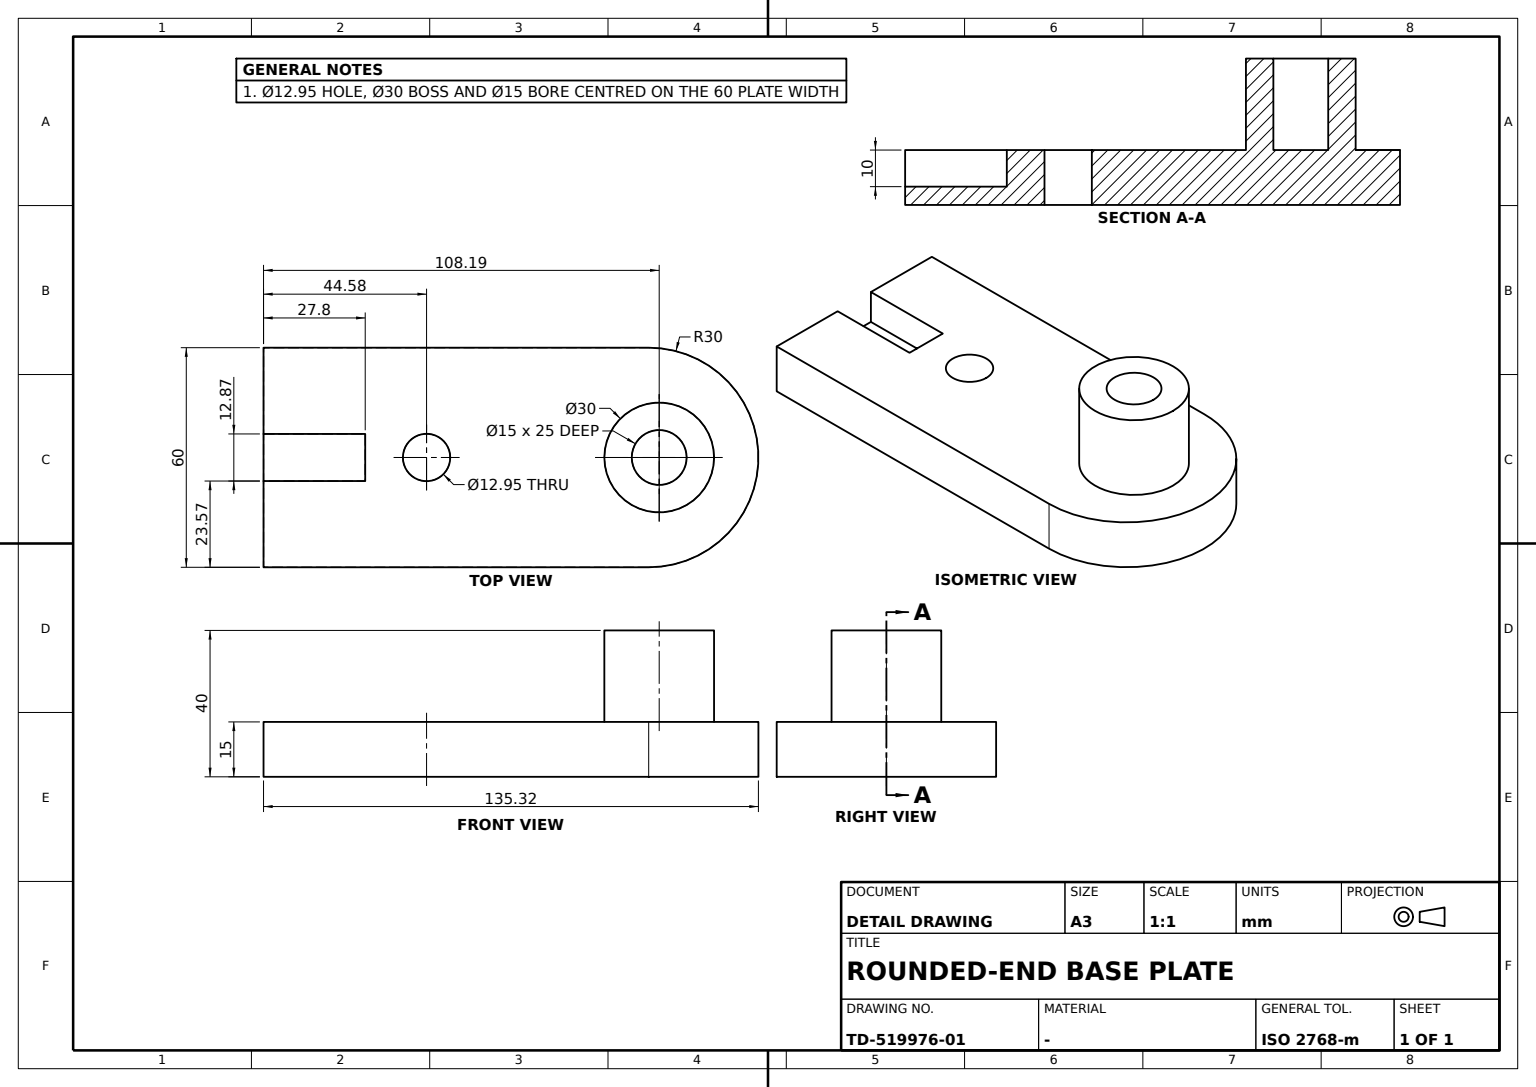
CATIA V5 part; units mm, degrees
sketch "Sketch1" plane through (0, 0, 0) normal (0, 0, 1) x (1, 0, 0)
  line L0 (40.1579, -30) -> (-65.1579, -30)
  line L1 (-65.1579, -30) -> (-65.1579, 30)
  line L2 (-65.1579, 30) -> (40.1579, 30)
  arc A0 (40.1579, 30) -> (40.1579, -30) centre (40.1579, 0) cw
  point P0 (40.1579, 30)
  point P1 (40.1579, -30)
  point P2 (40.1579, -30)
  point P3 (40.1579, 30)
  dimension "length L1" = 60
  constraint horizontal L0 x-axis
  constraint horizontal L2 x-axis
  constraint vertical L1 y-axis
  constraint equidistance L0 L2 origin
  constraint coincidence P0 L2
  constraint coincidence P1 L0
  constraint coincidence P0 P3
  constraint coincidence P1 P2
  constraint tangency A0 L0
extrude "Pad1" add sketch "Sketch1" along normal blind 15
sketch "Sketch2" plane through (0, 0, 15) normal (0, 0, 1) x (1, 0, 0)
  line L0 (43.0311, 28.8591) -> (43.0311, -47.18) construction
  circle A0 centre (43.0311, 0) radius 15
  point P0 (43.0311, 0)
  circle A1 centre (43.0311, 0) radius 7.5
  point P1 (50.5311, 0)
  dimension "radius A0" = 15
  dimension "radius A1" = 7.5
  constraint vertical L0 y-axis
  constraint coincidence P0 L0
  constraint coincidence P0 x-axis
  constraint coincidence A1 P1
  constraint coincidence P1 x-axis
extrude "Pad2" add sketch "Sketch2" along normal blind 25
sketch "Sketch3" plane through (0, 0, 15) normal (0, 0, 1) x (1, 0, 0)
  point P0 (-64.9666, 0)
  line L0 (-37.3555, 6.4328) -> (-37.3555, -6.4328)
  line L1 (-37.3555, -6.4328) -> (-92.5776, -6.4328)
  line L2 (-92.5776, -6.4328) -> (-92.5776, 6.4328)
  line L3 (-92.5776, 6.4328) -> (-37.3555, 6.4328)
  constraint coincidence P0 x-axis
  constraint vertical L0 y-axis
  constraint vertical L2 y-axis
  constraint horizontal L1 x-axis
  constraint horizontal L3 x-axis
  constraint equidistance L0 L2 P0
  constraint equidistance L1 L3 P0
extrude "Pocket1" cut sketch "Sketch3" against normal blind 10
sketch "Sketch4" plane through (0, 0, 15) normal (0, 0, 1) x (1, 0, 0)
  circle A0 centre (-20.5792, 0) radius 6.4738
  point P0 (-20.5792, 0)
  constraint coincidence P0 x-axis
extrude "Pocket2" cut sketch "Sketch4" against normal through all
